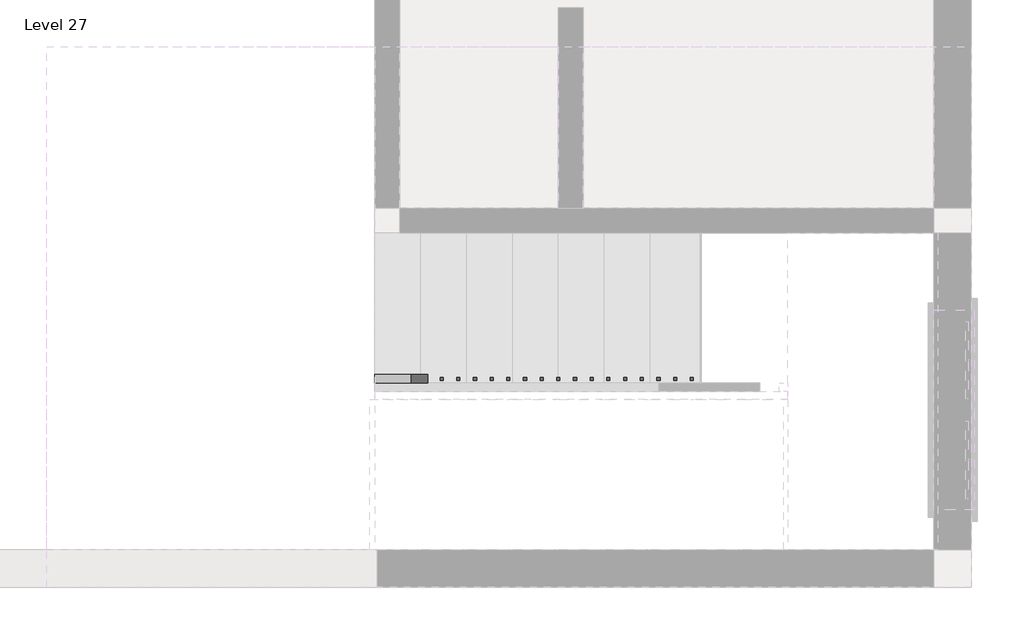
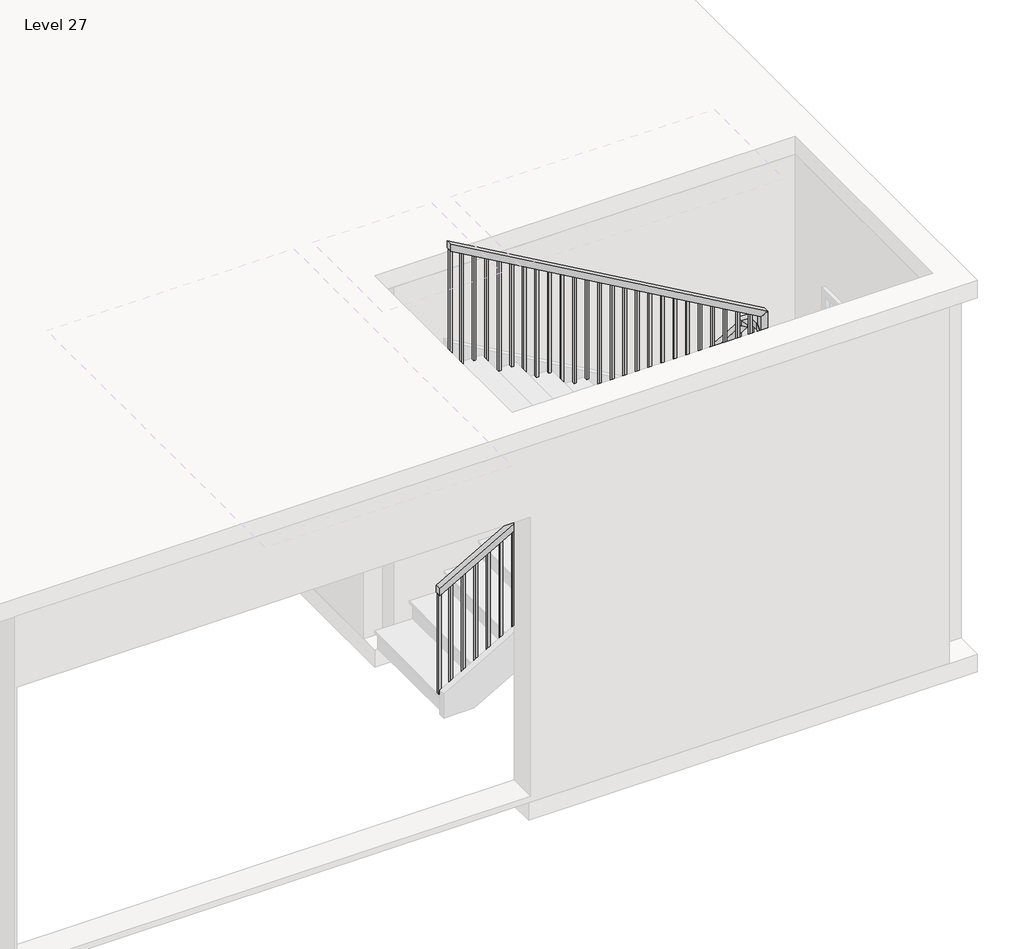
# One storey, part 2 of 3: 2 railings.
"""IFC4 building model written with IfcOpenShell, lengths in millimetres."""

from ifc_helpers import new_model, si_unit, frame, origin, place, context, project, spatial, polyline, outline, extrude, faceted_brep, element, save

model = new_model("IFC4")

# Units and contexts
model_context = context("Model", 3, world=origin())
ifc_project = project(units=[si_unit("LENGTHUNIT", "METRE", prefix="MILLI")], contexts=[model_context])

# Site, building, storey
site = spatial("IfcSite", under=ifc_project)
building = spatial("IfcBuilding", under=site)
storey = spatial("IfcBuildingStorey", under=building, Name="Level 27", Elevation=22402.8)

# Railings
placement = place(None, origin())
element("IfcRailing", 1, ObjectType="Handrail - Rectangular", at=placement, inside=storey, context=model_context, shape_type="SolidModel", body=[
    faceted_brep([(-1591.1154463, -4686.5544725, 23477.22), (-1591.1154463, -4686.5544725, 23418.6782835), (-1591.1154463, -4737.3544725, 23418.6782835), (-1591.1154463, -4737.3544725, 23477.22), (847.2845537, -4686.5544725, 24873.7581818), (898.0845537, -4686.5544725, 24844.3110107), (898.0845537, -4737.3544725, 24844.3110107), (847.2845537, -4737.3544725, 24873.7581818), (847.2845537, -4686.5544725, 24917.4), (898.0845537, -4686.5544725, 24866.6), (898.0845537, -4737.3544725, 24866.6), (847.2845537, -4737.3544725, 24917.4), (974.2845537, -4686.5544725, 24917.4), (974.2845537, -4686.5544725, 24866.6), (923.4845537, -4737.3544725, 24866.6), (923.4845537, -4737.3544725, 24917.4), (974.2845537, -4813.5544725, 24917.4), (974.2845537, -4813.5544725, 24866.6), (923.4845537, -4813.5544725, 24866.6), (923.4845537, -4813.5544725, 24917.4), (974.2845537, -4838.9544725, 24917.4), (923.4845537, -4838.9544725, 24917.4), (923.4845537, -4889.7544725, 24866.6), (974.2845537, -4889.7544725, 24866.6)], [[[0, 1, 2, 3]], [[1, 0, 4, 5]], [[2, 1, 5, 6]], [[3, 2, 6, 7]], [[0, 3, 7, 4]], [[5, 4, 8, 9]], [[6, 5, 9, 10]], [[7, 6, 10, 11]], [[4, 7, 11, 8]], [[9, 8, 12, 13]], [[10, 9, 13, 14]], [[11, 10, 14, 15]], [[8, 11, 15, 12]], [[13, 12, 16, 17]], [[14, 13, 17, 18]], [[15, 14, 18, 19]], [[12, 15, 19, 16]], [[20, 21, 22, 23]], [[17, 16, 20, 23]], [[18, 17, 23, 22]], [[19, 18, 22, 21]], [[16, 19, 21, 20]]]),
    faceted_brep([(974.2845537, -4838.9544725, 24917.4), (974.2845537, -4889.7544725, 24866.6), (923.4845537, -4889.7544725, 24866.6), (923.4845537, -4838.9544725, 24917.4), (974.2845537, -4838.9544725, 25048.3254545), (923.4845537, -4838.9544725, 25018.8782835), (923.4845537, -4889.7544725, 25018.8782835), (974.2845537, -4889.7544725, 25048.3254545)], [[[0, 1, 2, 3]], [[4, 5, 6, 7]], [[1, 0, 4, 7]], [[2, 1, 7, 6]], [[3, 2, 6, 5]], [[0, 3, 5, 4]]]),
    faceted_brep([(974.2845537, -4889.7544725, 25048.3254545), (923.4845537, -4889.7544725, 25018.8782835), (923.4845537, -4838.9544725, 25018.8782835), (974.2845537, -4838.9544725, 25048.3254545), (-1591.1154463, -4889.7544725, 26517.6), (-1591.1154463, -4838.9544725, 26517.6), (-1591.1154463, -4838.9544725, 26459.0582835), (-1591.1154463, -4889.7544725, 26459.0582835)], [[[0, 1, 2, 3]], [[4, 5, 6, 7]], [[1, 0, 4, 7]], [[2, 1, 7, 6]], [[3, 2, 6, 5]], [[0, 3, 5, 4]]]),
    extrude(outline(polyline([(26395.4139653, -1479.9904463), (26406.3244198, -1499.0404463), (25443.18, -1499.0404463), (25443.18, -1479.9904463), (26395.4139653, -1479.9904463)])), frame((0.0, -4873.8794725, 0.0), z_axis=(0.0, 1.0, 0.0), x_axis=(0.0, 0.0, 1.0)), (0.0, 0.0, 1.0), 19.05),
    extrude(outline(polyline([(26337.2248744, -1378.3904463), (26348.1353289, -1397.4404463), (25443.18, -1397.4404463), (25443.18, -1378.3904463), (26337.2248744, -1378.3904463)])), frame((0.0, -4873.8794725, 0.0), z_axis=(0.0, 1.0, 0.0), x_axis=(0.0, 0.0, 1.0)), (0.0, 0.0, 1.0), 19.05),
    extrude(outline(polyline([(26279.0357835, -1276.7904463), (26289.946238, -1295.8404463), (25283.16, -1295.8404463), (25283.16, -1276.7904463), (26279.0357835, -1276.7904463)])), frame((0.0, -4873.8794725, 0.0), z_axis=(0.0, 1.0, 0.0), x_axis=(0.0, 0.0, 1.0)), (0.0, 0.0, 1.0), 19.05),
    extrude(outline(polyline([(26220.8466926, -1175.1904463), (26231.7571471, -1194.2404463), (25283.16, -1194.2404463), (25283.16, -1175.1904463), (26220.8466926, -1175.1904463)])), frame((0.0, -4873.8794725, 0.0), z_axis=(0.0, 1.0, 0.0), x_axis=(0.0, 0.0, 1.0)), (0.0, 0.0, 1.0), 19.05),
    extrude(outline(polyline([(26162.6576016, -1073.5904463), (26173.5680562, -1092.6404463), (25283.16, -1092.6404463), (25283.16, -1073.5904463), (26162.6576016, -1073.5904463)])), frame((0.0, -4873.8794725, 0.0), z_axis=(0.0, 1.0, 0.0), x_axis=(0.0, 0.0, 1.0)), (0.0, 0.0, 1.0), 19.05),
    extrude(outline(polyline([(26104.4685107, -971.9904463), (26115.3789653, -991.0404463), (25123.14, -991.0404463), (25123.14, -971.9904463), (26104.4685107, -971.9904463)])), frame((0.0, -4873.8794725, 0.0), z_axis=(0.0, 1.0, 0.0), x_axis=(0.0, 0.0, 1.0)), (0.0, 0.0, 1.0), 19.05),
    extrude(outline(polyline([(26046.2794198, -870.3904463), (26057.1898744, -889.4404463), (25123.14, -889.4404463), (25123.14, -870.3904463), (26046.2794198, -870.3904463)])), frame((0.0, -4873.8794725, 0.0), z_axis=(0.0, 1.0, 0.0), x_axis=(0.0, 0.0, 1.0)), (0.0, 0.0, 1.0), 19.05),
    extrude(outline(polyline([(25988.0903289, -768.7904463), (25999.0007835, -787.8404463), (25123.14, -787.8404463), (25123.14, -768.7904463), (25988.0903289, -768.7904463)])), frame((0.0, -4873.8794725, 0.0), z_axis=(0.0, 1.0, 0.0), x_axis=(0.0, 0.0, 1.0)), (0.0, 0.0, 1.0), 19.05),
    extrude(outline(polyline([(25929.901238, -667.1904463), (25940.8116926, -686.2404463), (24963.12, -686.2404463), (24963.12, -667.1904463), (25929.901238, -667.1904463)])), frame((0.0, -4873.8794725, 0.0), z_axis=(0.0, 1.0, 0.0), x_axis=(0.0, 0.0, 1.0)), (0.0, 0.0, 1.0), 19.05),
    extrude(outline(polyline([(25871.7121471, -565.5904463), (25882.6226016, -584.6404463), (24963.12, -584.6404463), (24963.12, -565.5904463), (25871.7121471, -565.5904463)])), frame((0.0, -4873.8794725, 0.0), z_axis=(0.0, 1.0, 0.0), x_axis=(0.0, 0.0, 1.0)), (0.0, 0.0, 1.0), 19.05),
    extrude(outline(polyline([(25813.5230562, -463.9904463), (25824.4335107, -483.0404463), (24963.12, -483.0404463), (24963.12, -463.9904463), (25813.5230562, -463.9904463)])), frame((0.0, -4873.8794725, 0.0), z_axis=(0.0, 1.0, 0.0), x_axis=(0.0, 0.0, 1.0)), (0.0, 0.0, 1.0), 19.05),
    extrude(outline(polyline([(25755.3339653, -362.3904463), (25766.2444198, -381.4404463), (24803.1, -381.4404463), (24803.1, -362.3904463), (25755.3339653, -362.3904463)])), frame((0.0, -4873.8794725, 0.0), z_axis=(0.0, 1.0, 0.0), x_axis=(0.0, 0.0, 1.0)), (0.0, 0.0, 1.0), 19.05),
    extrude(outline(polyline([(25697.1448744, -260.7904463), (25708.0553289, -279.8404463), (24803.1, -279.8404463), (24803.1, -260.7904463), (25697.1448744, -260.7904463)])), frame((0.0, -4873.8794725, 0.0), z_axis=(0.0, 1.0, 0.0), x_axis=(0.0, 0.0, 1.0)), (0.0, 0.0, 1.0), 19.05),
    extrude(outline(polyline([(25638.9557835, -159.1904463), (25649.866238, -178.2404463), (24643.08, -178.2404463), (24643.08, -159.1904463), (25638.9557835, -159.1904463)])), frame((0.0, -4873.8794725, 0.0), z_axis=(0.0, 1.0, 0.0), x_axis=(0.0, 0.0, 1.0)), (0.0, 0.0, 1.0), 19.05),
    extrude(outline(polyline([(25580.7666926, -57.5904463), (25591.6771471, -76.6404463), (24643.08, -76.6404463), (24643.08, -57.5904463), (25580.7666926, -57.5904463)])), frame((0.0, -4873.8794725, 0.0), z_axis=(0.0, 1.0, 0.0), x_axis=(0.0, 0.0, 1.0)), (0.0, 0.0, 1.0), 19.05),
    extrude(outline(polyline([(25522.5776016, 44.0095537), (25533.4880562, 24.9595537), (24643.08, 24.9595537), (24643.08, 44.0095537), (25522.5776016, 44.0095537)])), frame((0.0, -4873.8794725, 0.0), z_axis=(0.0, 1.0, 0.0), x_axis=(0.0, 0.0, 1.0)), (0.0, 0.0, 1.0), 19.05),
    extrude(outline(polyline([(25464.3885107, 145.6095537), (25475.2989653, 126.5595537), (24483.06, 126.5595537), (24483.06, 145.6095537), (25464.3885107, 145.6095537)])), frame((0.0, -4873.8794725, 0.0), z_axis=(0.0, 1.0, 0.0), x_axis=(0.0, 0.0, 1.0)), (0.0, 0.0, 1.0), 19.05),
    extrude(outline(polyline([(25406.1994198, 247.2095537), (25417.1098744, 228.1595537), (24483.06, 228.1595537), (24483.06, 247.2095537), (25406.1994198, 247.2095537)])), frame((0.0, -4873.8794725, 0.0), z_axis=(0.0, 1.0, 0.0), x_axis=(0.0, 0.0, 1.0)), (0.0, 0.0, 1.0), 19.05),
    extrude(outline(polyline([(25348.0103289, 348.8095537), (25358.9207835, 329.7595537), (24483.06, 329.7595537), (24483.06, 348.8095537), (25348.0103289, 348.8095537)])), frame((0.0, -4873.8794725, 0.0), z_axis=(0.0, 1.0, 0.0), x_axis=(0.0, 0.0, 1.0)), (0.0, 0.0, 1.0), 19.05),
    extrude(outline(polyline([(25289.821238, 450.4095537), (25300.7316926, 431.3595537), (24323.04, 431.3595537), (24323.04, 450.4095537), (25289.821238, 450.4095537)])), frame((0.0, -4873.8794725, 0.0), z_axis=(0.0, 1.0, 0.0), x_axis=(0.0, 0.0, 1.0)), (0.0, 0.0, 1.0), 19.05),
    extrude(outline(polyline([(25231.6321471, 552.0095537), (25242.5426016, 532.9595537), (24323.04, 532.9595537), (24323.04, 552.0095537), (25231.6321471, 552.0095537)])), frame((0.0, -4873.8794725, 0.0), z_axis=(0.0, 1.0, 0.0), x_axis=(0.0, 0.0, 1.0)), (0.0, 0.0, 1.0), 19.05),
    extrude(outline(polyline([(25173.4430562, 653.6095537), (25184.3535107, 634.5595537), (24323.04, 634.5595537), (24323.04, 653.6095537), (25173.4430562, 653.6095537)])), frame((0.0, -4873.8794725, 0.0), z_axis=(0.0, 1.0, 0.0), x_axis=(0.0, 0.0, 1.0)), (0.0, 0.0, 1.0), 19.05),
    extrude(outline(polyline([(25115.2539653, 755.2095537), (25126.1644198, 736.1595537), (24163.02, 736.1595537), (24163.02, 755.2095537), (25115.2539653, 755.2095537)])), frame((0.0, -4873.8794725, 0.0), z_axis=(0.0, 1.0, 0.0), x_axis=(0.0, 0.0, 1.0)), (0.0, 0.0, 1.0), 19.05),
    extrude(outline(polyline([(25057.0648744, 856.8095537), (25067.9753289, 837.7595537), (24163.02, 837.7595537), (24163.02, 856.8095537), (25057.0648744, 856.8095537)])), frame((0.0, -4873.8794725, 0.0), z_axis=(0.0, 1.0, 0.0), x_axis=(0.0, 0.0, 1.0)), (0.0, 0.0, 1.0), 19.05),
    extrude(outline(polyline([(939.3595537, -4804.0294725), (958.4095537, -4804.0294725), (958.4095537, -4823.0794725), (939.3595537, -4823.0794725), (939.3595537, -4804.0294725)])), frame((0.0, 0.0, 24003.0), z_axis=(0.0, 0.0, 1.0), x_axis=(1.0, 0.0, 0.0)), (0.0, 0.0, 1.0), 863.6),
    extrude(outline(polyline([(24820.6716926, 856.8095537), (24809.761238, 837.7595537), (23842.98, 837.7595537), (23842.98, 856.8095537), (24820.6716926, 856.8095537)])), frame((0.0, -4721.4794725, 0.0), z_axis=(0.0, 1.0, 0.0), x_axis=(0.0, 0.0, 1.0)), (0.0, 0.0, 1.0), 19.05),
    extrude(outline(polyline([(24762.4826016, 755.2095537), (24751.5721471, 736.1595537), (23842.98, 736.1595537), (23842.98, 755.2095537), (24762.4826016, 755.2095537)])), frame((0.0, -4721.4794725, 0.0), z_axis=(0.0, 1.0, 0.0), x_axis=(0.0, 0.0, 1.0)), (0.0, 0.0, 1.0), 19.05),
    extrude(outline(polyline([(24704.2935107, 653.6095537), (24693.3830562, 634.5595537), (23842.98, 634.5595537), (23842.98, 653.6095537), (24704.2935107, 653.6095537)])), frame((0.0, -4721.4794725, 0.0), z_axis=(0.0, 1.0, 0.0), x_axis=(0.0, 0.0, 1.0)), (0.0, 0.0, 1.0), 19.05),
    extrude(outline(polyline([(24646.1044198, 552.0095537), (24635.1939653, 532.9595537), (23682.96, 532.9595537), (23682.96, 552.0095537), (24646.1044198, 552.0095537)])), frame((0.0, -4721.4794725, 0.0), z_axis=(0.0, 1.0, 0.0), x_axis=(0.0, 0.0, 1.0)), (0.0, 0.0, 1.0), 19.05),
    extrude(outline(polyline([(24587.9153289, 450.4095537), (24577.0048744, 431.3595537), (23682.96, 431.3595537), (23682.96, 450.4095537), (24587.9153289, 450.4095537)])), frame((0.0, -4721.4794725, 0.0), z_axis=(0.0, 1.0, 0.0), x_axis=(0.0, 0.0, 1.0)), (0.0, 0.0, 1.0), 19.05),
    extrude(outline(polyline([(24529.726238, 348.8095537), (24518.8157835, 329.7595537), (23522.94, 329.7595537), (23522.94, 348.8095537), (24529.726238, 348.8095537)])), frame((0.0, -4721.4794725, 0.0), z_axis=(0.0, 1.0, 0.0), x_axis=(0.0, 0.0, 1.0)), (0.0, 0.0, 1.0), 19.05),
    extrude(outline(polyline([(24471.5371471, 247.2095537), (24460.6266926, 228.1595537), (23522.94, 228.1595537), (23522.94, 247.2095537), (24471.5371471, 247.2095537)])), frame((0.0, -4721.4794725, 0.0), z_axis=(0.0, 1.0, 0.0), x_axis=(0.0, 0.0, 1.0)), (0.0, 0.0, 1.0), 19.05),
    extrude(outline(polyline([(24413.3480562, 145.6095537), (24402.4376016, 126.5595537), (23522.94, 126.5595537), (23522.94, 145.6095537), (24413.3480562, 145.6095537)])), frame((0.0, -4721.4794725, 0.0), z_axis=(0.0, 1.0, 0.0), x_axis=(0.0, 0.0, 1.0)), (0.0, 0.0, 1.0), 19.05),
    extrude(outline(polyline([(24355.1589653, 44.0095537), (24344.2485107, 24.9595537), (23362.92, 24.9595537), (23362.92, 44.0095537), (24355.1589653, 44.0095537)])), frame((0.0, -4721.4794725, 0.0), z_axis=(0.0, 1.0, 0.0), x_axis=(0.0, 0.0, 1.0)), (0.0, 0.0, 1.0), 19.05),
    extrude(outline(polyline([(24296.9698744, -57.5904463), (24286.0594198, -76.6404463), (23362.92, -76.6404463), (23362.92, -57.5904463), (24296.9698744, -57.5904463)])), frame((0.0, -4721.4794725, 0.0), z_axis=(0.0, 1.0, 0.0), x_axis=(0.0, 0.0, 1.0)), (0.0, 0.0, 1.0), 19.05),
    extrude(outline(polyline([(24238.7807835, -159.1904463), (24227.8703289, -178.2404463), (23362.92, -178.2404463), (23362.92, -159.1904463), (24238.7807835, -159.1904463)])), frame((0.0, -4721.4794725, 0.0), z_axis=(0.0, 1.0, 0.0), x_axis=(0.0, 0.0, 1.0)), (0.0, 0.0, 1.0), 19.05),
    extrude(outline(polyline([(24180.5916926, -260.7904463), (24169.681238, -279.8404463), (23202.9, -279.8404463), (23202.9, -260.7904463), (24180.5916926, -260.7904463)])), frame((0.0, -4721.4794725, 0.0), z_axis=(0.0, 1.0, 0.0), x_axis=(0.0, 0.0, 1.0)), (0.0, 0.0, 1.0), 19.05),
    extrude(outline(polyline([(24122.4026016, -362.3904463), (24111.4921471, -381.4404463), (23202.9, -381.4404463), (23202.9, -362.3904463), (24122.4026016, -362.3904463)])), frame((0.0, -4721.4794725, 0.0), z_axis=(0.0, 1.0, 0.0), x_axis=(0.0, 0.0, 1.0)), (0.0, 0.0, 1.0), 19.05),
    extrude(outline(polyline([(24064.2135107, -463.9904463), (24053.3030562, -483.0404463), (23202.9, -483.0404463), (23202.9, -463.9904463), (24064.2135107, -463.9904463)])), frame((0.0, -4721.4794725, 0.0), z_axis=(0.0, 1.0, 0.0), x_axis=(0.0, 0.0, 1.0)), (0.0, 0.0, 1.0), 19.05),
    extrude(outline(polyline([(24006.0244198, -565.5904463), (23995.1139653, -584.6404463), (23042.88, -584.6404463), (23042.88, -565.5904463), (24006.0244198, -565.5904463)])), frame((0.0, -4721.4794725, 0.0), z_axis=(0.0, 1.0, 0.0), x_axis=(0.0, 0.0, 1.0)), (0.0, 0.0, 1.0), 19.05),
    extrude(outline(polyline([(23947.8353289, -667.1904463), (23936.9248744, -686.2404463), (23042.88, -686.2404463), (23042.88, -667.1904463), (23947.8353289, -667.1904463)])), frame((0.0, -4721.4794725, 0.0), z_axis=(0.0, 1.0, 0.0), x_axis=(0.0, 0.0, 1.0)), (0.0, 0.0, 1.0), 19.05),
    extrude(outline(polyline([(23889.646238, -768.7904463), (23878.7357835, -787.8404463), (22882.86, -787.8404463), (22882.86, -768.7904463), (23889.646238, -768.7904463)])), frame((0.0, -4721.4794725, 0.0), z_axis=(0.0, 1.0, 0.0), x_axis=(0.0, 0.0, 1.0)), (0.0, 0.0, 1.0), 19.05),
    extrude(outline(polyline([(23831.4571471, -870.3904463), (23820.5466926, -889.4404463), (22882.86, -889.4404463), (22882.86, -870.3904463), (23831.4571471, -870.3904463)])), frame((0.0, -4721.4794725, 0.0), z_axis=(0.0, 1.0, 0.0), x_axis=(0.0, 0.0, 1.0)), (0.0, 0.0, 1.0), 19.05),
    extrude(outline(polyline([(23773.2680562, -971.9904463), (23762.3576016, -991.0404463), (22882.86, -991.0404463), (22882.86, -971.9904463), (23773.2680562, -971.9904463)])), frame((0.0, -4721.4794725, 0.0), z_axis=(0.0, 1.0, 0.0), x_axis=(0.0, 0.0, 1.0)), (0.0, 0.0, 1.0), 19.05),
    extrude(outline(polyline([(23715.0789653, -1073.5904463), (23704.1685107, -1092.6404463), (22722.84, -1092.6404463), (22722.84, -1073.5904463), (23715.0789653, -1073.5904463)])), frame((0.0, -4721.4794725, 0.0), z_axis=(0.0, 1.0, 0.0), x_axis=(0.0, 0.0, 1.0)), (0.0, 0.0, 1.0), 19.05),
    extrude(outline(polyline([(23656.8898744, -1175.1904463), (23645.9794198, -1194.2404463), (22722.84, -1194.2404463), (22722.84, -1175.1904463), (23656.8898744, -1175.1904463)])), frame((0.0, -4721.4794725, 0.0), z_axis=(0.0, 1.0, 0.0), x_axis=(0.0, 0.0, 1.0)), (0.0, 0.0, 1.0), 19.05),
    extrude(outline(polyline([(23598.7007835, -1276.7904463), (23587.7903289, -1295.8404463), (22722.84, -1295.8404463), (22722.84, -1276.7904463), (23598.7007835, -1276.7904463)])), frame((0.0, -4721.4794725, 0.0), z_axis=(0.0, 1.0, 0.0), x_axis=(0.0, 0.0, 1.0)), (0.0, 0.0, 1.0), 19.05),
    extrude(outline(polyline([(23540.5116926, -1378.3904463), (23529.601238, -1397.4404463), (22562.82, -1397.4404463), (22562.82, -1378.3904463), (23540.5116926, -1378.3904463)])), frame((0.0, -4721.4794725, 0.0), z_axis=(0.0, 1.0, 0.0), x_axis=(0.0, 0.0, 1.0)), (0.0, 0.0, 1.0), 19.05),
    extrude(outline(polyline([(23482.3226016, -1479.9904463), (23471.4121471, -1499.0404463), (22562.82, -1499.0404463), (22562.82, -1479.9904463), (23482.3226016, -1479.9904463)])), frame((0.0, -4721.4794725, 0.0), z_axis=(0.0, 1.0, 0.0), x_axis=(0.0, 0.0, 1.0)), (0.0, 0.0, 1.0), 19.05),
    extrude(outline(polyline([(939.3595537, -4854.8294725), (958.4095537, -4854.8294725), (958.4095537, -4873.8794725), (939.3595537, -4873.8794725), (939.3595537, -4854.8294725)])), frame((0.0, 0.0, 24003.0), z_axis=(0.0, 0.0, 1.0), x_axis=(1.0, 0.0, 0.0)), (0.0, 0.0, 1.0), 863.6),
    extrude(outline(polyline([(939.3595537, -4721.4794725), (939.3595537, -4702.4294725), (958.4095537, -4702.4294725), (958.4095537, -4721.4794725), (939.3595537, -4721.4794725)])), frame((0.0, 0.0, 24003.0), z_axis=(0.0, 0.0, 1.0), x_axis=(1.0, 0.0, 0.0)), (0.0, 0.0, 1.0), 863.6),
    extrude(outline(polyline([(26448.1478289, -1572.0654463), (26459.0582835, -1591.1154463), (25443.18, -1591.1154463), (25443.18, -1572.0654463), (26448.1478289, -1572.0654463)])), frame((0.0, -4873.8794725, 0.0), z_axis=(0.0, 1.0, 0.0), x_axis=(0.0, 0.0, 1.0)), (0.0, 0.0, 1.0), 19.05),
    extrude(outline(polyline([(23429.588738, -1572.0654463), (23418.6782835, -1591.1154463), (22562.82, -1591.1154463), (22562.82, -1572.0654463), (23429.588738, -1572.0654463)])), frame((0.0, -4721.4794725, 0.0), z_axis=(0.0, 1.0, 0.0), x_axis=(0.0, 0.0, 1.0)), (0.0, 0.0, 1.0), 19.05),
])
element("IfcRailing", 2, ObjectType="Handrail - Rectangular", at=placement, inside=storey, context=model_context, shape_type="SolidModel", body=[
    faceted_brep([(-1591.1154463, -4686.5544725, 23477.22), (-1591.1154463, -4686.5544725, 23418.6782835), (-1591.1154463, -4737.3544725, 23418.6782835), (-1591.1154463, -4737.3544725, 23477.22), (847.2845537, -4686.5544725, 24873.7581818), (898.0845537, -4686.5544725, 24844.3110107), (898.0845537, -4737.3544725, 24844.3110107), (847.2845537, -4737.3544725, 24873.7581818), (847.2845537, -4686.5544725, 24917.4), (898.0845537, -4686.5544725, 24866.6), (898.0845537, -4737.3544725, 24866.6), (847.2845537, -4737.3544725, 24917.4), (974.2845537, -4686.5544725, 24917.4), (974.2845537, -4686.5544725, 24866.6), (923.4845537, -4737.3544725, 24866.6), (923.4845537, -4737.3544725, 24917.4), (974.2845537, -4813.5544725, 24917.4), (974.2845537, -4813.5544725, 24866.6), (923.4845537, -4813.5544725, 24866.6), (923.4845537, -4813.5544725, 24917.4), (974.2845537, -4838.9544725, 24917.4), (923.4845537, -4838.9544725, 24917.4), (923.4845537, -4889.7544725, 24866.6), (974.2845537, -4889.7544725, 24866.6)], [[[0, 1, 2, 3]], [[1, 0, 4, 5]], [[2, 1, 5, 6]], [[3, 2, 6, 7]], [[0, 3, 7, 4]], [[5, 4, 8, 9]], [[6, 5, 9, 10]], [[7, 6, 10, 11]], [[4, 7, 11, 8]], [[9, 8, 12, 13]], [[10, 9, 13, 14]], [[11, 10, 14, 15]], [[8, 11, 15, 12]], [[13, 12, 16, 17]], [[14, 13, 17, 18]], [[15, 14, 18, 19]], [[12, 15, 19, 16]], [[20, 21, 22, 23]], [[17, 16, 20, 23]], [[18, 17, 23, 22]], [[19, 18, 22, 21]], [[16, 19, 21, 20]]]),
    faceted_brep([(974.2845537, -4838.9544725, 24917.4), (974.2845537, -4889.7544725, 24866.6), (923.4845537, -4889.7544725, 24866.6), (923.4845537, -4838.9544725, 24917.4), (974.2845537, -4838.9544725, 25048.3254545), (923.4845537, -4838.9544725, 25018.8782835), (923.4845537, -4889.7544725, 25018.8782835), (974.2845537, -4889.7544725, 25048.3254545)], [[[0, 1, 2, 3]], [[4, 5, 6, 7]], [[1, 0, 4, 7]], [[2, 1, 7, 6]], [[3, 2, 6, 5]], [[0, 3, 5, 4]]]),
    faceted_brep([(974.2845537, -4889.7544725, 25048.3254545), (923.4845537, -4889.7544725, 25018.8782835), (923.4845537, -4838.9544725, 25018.8782835), (974.2845537, -4838.9544725, 25048.3254545), (-1591.1154463, -4889.7544725, 26517.6), (-1591.1154463, -4838.9544725, 26517.6), (-1591.1154463, -4838.9544725, 26459.0582835), (-1591.1154463, -4889.7544725, 26459.0582835)], [[[0, 1, 2, 3]], [[4, 5, 6, 7]], [[1, 0, 4, 7]], [[2, 1, 7, 6]], [[3, 2, 6, 5]], [[0, 3, 5, 4]]]),
    extrude(outline(polyline([(26395.4139653, -1479.9904463), (26406.3244198, -1499.0404463), (25443.18, -1499.0404463), (25443.18, -1479.9904463), (26395.4139653, -1479.9904463)])), frame((0.0, -4873.8794725, 0.0), z_axis=(0.0, 1.0, 0.0), x_axis=(0.0, 0.0, 1.0)), (0.0, 0.0, 1.0), 19.05),
    extrude(outline(polyline([(26337.2248744, -1378.3904463), (26348.1353289, -1397.4404463), (25443.18, -1397.4404463), (25443.18, -1378.3904463), (26337.2248744, -1378.3904463)])), frame((0.0, -4873.8794725, 0.0), z_axis=(0.0, 1.0, 0.0), x_axis=(0.0, 0.0, 1.0)), (0.0, 0.0, 1.0), 19.05),
    extrude(outline(polyline([(26279.0357835, -1276.7904463), (26289.946238, -1295.8404463), (25283.16, -1295.8404463), (25283.16, -1276.7904463), (26279.0357835, -1276.7904463)])), frame((0.0, -4873.8794725, 0.0), z_axis=(0.0, 1.0, 0.0), x_axis=(0.0, 0.0, 1.0)), (0.0, 0.0, 1.0), 19.05),
    extrude(outline(polyline([(26220.8466926, -1175.1904463), (26231.7571471, -1194.2404463), (25283.16, -1194.2404463), (25283.16, -1175.1904463), (26220.8466926, -1175.1904463)])), frame((0.0, -4873.8794725, 0.0), z_axis=(0.0, 1.0, 0.0), x_axis=(0.0, 0.0, 1.0)), (0.0, 0.0, 1.0), 19.05),
    extrude(outline(polyline([(26162.6576016, -1073.5904463), (26173.5680562, -1092.6404463), (25283.16, -1092.6404463), (25283.16, -1073.5904463), (26162.6576016, -1073.5904463)])), frame((0.0, -4873.8794725, 0.0), z_axis=(0.0, 1.0, 0.0), x_axis=(0.0, 0.0, 1.0)), (0.0, 0.0, 1.0), 19.05),
    extrude(outline(polyline([(26104.4685107, -971.9904463), (26115.3789653, -991.0404463), (25123.14, -991.0404463), (25123.14, -971.9904463), (26104.4685107, -971.9904463)])), frame((0.0, -4873.8794725, 0.0), z_axis=(0.0, 1.0, 0.0), x_axis=(0.0, 0.0, 1.0)), (0.0, 0.0, 1.0), 19.05),
    extrude(outline(polyline([(26046.2794198, -870.3904463), (26057.1898744, -889.4404463), (25123.14, -889.4404463), (25123.14, -870.3904463), (26046.2794198, -870.3904463)])), frame((0.0, -4873.8794725, 0.0), z_axis=(0.0, 1.0, 0.0), x_axis=(0.0, 0.0, 1.0)), (0.0, 0.0, 1.0), 19.05),
    extrude(outline(polyline([(25988.0903289, -768.7904463), (25999.0007835, -787.8404463), (25123.14, -787.8404463), (25123.14, -768.7904463), (25988.0903289, -768.7904463)])), frame((0.0, -4873.8794725, 0.0), z_axis=(0.0, 1.0, 0.0), x_axis=(0.0, 0.0, 1.0)), (0.0, 0.0, 1.0), 19.05),
    extrude(outline(polyline([(25929.901238, -667.1904463), (25940.8116926, -686.2404463), (24963.12, -686.2404463), (24963.12, -667.1904463), (25929.901238, -667.1904463)])), frame((0.0, -4873.8794725, 0.0), z_axis=(0.0, 1.0, 0.0), x_axis=(0.0, 0.0, 1.0)), (0.0, 0.0, 1.0), 19.05),
    extrude(outline(polyline([(25871.7121471, -565.5904463), (25882.6226016, -584.6404463), (24963.12, -584.6404463), (24963.12, -565.5904463), (25871.7121471, -565.5904463)])), frame((0.0, -4873.8794725, 0.0), z_axis=(0.0, 1.0, 0.0), x_axis=(0.0, 0.0, 1.0)), (0.0, 0.0, 1.0), 19.05),
    extrude(outline(polyline([(25813.5230562, -463.9904463), (25824.4335107, -483.0404463), (24963.12, -483.0404463), (24963.12, -463.9904463), (25813.5230562, -463.9904463)])), frame((0.0, -4873.8794725, 0.0), z_axis=(0.0, 1.0, 0.0), x_axis=(0.0, 0.0, 1.0)), (0.0, 0.0, 1.0), 19.05),
    extrude(outline(polyline([(25755.3339653, -362.3904463), (25766.2444198, -381.4404463), (24803.1, -381.4404463), (24803.1, -362.3904463), (25755.3339653, -362.3904463)])), frame((0.0, -4873.8794725, 0.0), z_axis=(0.0, 1.0, 0.0), x_axis=(0.0, 0.0, 1.0)), (0.0, 0.0, 1.0), 19.05),
    extrude(outline(polyline([(25697.1448744, -260.7904463), (25708.0553289, -279.8404463), (24803.1, -279.8404463), (24803.1, -260.7904463), (25697.1448744, -260.7904463)])), frame((0.0, -4873.8794725, 0.0), z_axis=(0.0, 1.0, 0.0), x_axis=(0.0, 0.0, 1.0)), (0.0, 0.0, 1.0), 19.05),
    extrude(outline(polyline([(25638.9557835, -159.1904463), (25649.866238, -178.2404463), (24643.08, -178.2404463), (24643.08, -159.1904463), (25638.9557835, -159.1904463)])), frame((0.0, -4873.8794725, 0.0), z_axis=(0.0, 1.0, 0.0), x_axis=(0.0, 0.0, 1.0)), (0.0, 0.0, 1.0), 19.05),
    extrude(outline(polyline([(25580.7666926, -57.5904463), (25591.6771471, -76.6404463), (24643.08, -76.6404463), (24643.08, -57.5904463), (25580.7666926, -57.5904463)])), frame((0.0, -4873.8794725, 0.0), z_axis=(0.0, 1.0, 0.0), x_axis=(0.0, 0.0, 1.0)), (0.0, 0.0, 1.0), 19.05),
    extrude(outline(polyline([(25522.5776016, 44.0095537), (25533.4880562, 24.9595537), (24643.08, 24.9595537), (24643.08, 44.0095537), (25522.5776016, 44.0095537)])), frame((0.0, -4873.8794725, 0.0), z_axis=(0.0, 1.0, 0.0), x_axis=(0.0, 0.0, 1.0)), (0.0, 0.0, 1.0), 19.05),
    extrude(outline(polyline([(25464.3885107, 145.6095537), (25475.2989653, 126.5595537), (24483.06, 126.5595537), (24483.06, 145.6095537), (25464.3885107, 145.6095537)])), frame((0.0, -4873.8794725, 0.0), z_axis=(0.0, 1.0, 0.0), x_axis=(0.0, 0.0, 1.0)), (0.0, 0.0, 1.0), 19.05),
    extrude(outline(polyline([(25406.1994198, 247.2095537), (25417.1098744, 228.1595537), (24483.06, 228.1595537), (24483.06, 247.2095537), (25406.1994198, 247.2095537)])), frame((0.0, -4873.8794725, 0.0), z_axis=(0.0, 1.0, 0.0), x_axis=(0.0, 0.0, 1.0)), (0.0, 0.0, 1.0), 19.05),
    extrude(outline(polyline([(25348.0103289, 348.8095537), (25358.9207835, 329.7595537), (24483.06, 329.7595537), (24483.06, 348.8095537), (25348.0103289, 348.8095537)])), frame((0.0, -4873.8794725, 0.0), z_axis=(0.0, 1.0, 0.0), x_axis=(0.0, 0.0, 1.0)), (0.0, 0.0, 1.0), 19.05),
    extrude(outline(polyline([(25289.821238, 450.4095537), (25300.7316926, 431.3595537), (24323.04, 431.3595537), (24323.04, 450.4095537), (25289.821238, 450.4095537)])), frame((0.0, -4873.8794725, 0.0), z_axis=(0.0, 1.0, 0.0), x_axis=(0.0, 0.0, 1.0)), (0.0, 0.0, 1.0), 19.05),
    extrude(outline(polyline([(25231.6321471, 552.0095537), (25242.5426016, 532.9595537), (24323.04, 532.9595537), (24323.04, 552.0095537), (25231.6321471, 552.0095537)])), frame((0.0, -4873.8794725, 0.0), z_axis=(0.0, 1.0, 0.0), x_axis=(0.0, 0.0, 1.0)), (0.0, 0.0, 1.0), 19.05),
    extrude(outline(polyline([(25173.4430562, 653.6095537), (25184.3535107, 634.5595537), (24323.04, 634.5595537), (24323.04, 653.6095537), (25173.4430562, 653.6095537)])), frame((0.0, -4873.8794725, 0.0), z_axis=(0.0, 1.0, 0.0), x_axis=(0.0, 0.0, 1.0)), (0.0, 0.0, 1.0), 19.05),
    extrude(outline(polyline([(25115.2539653, 755.2095537), (25126.1644198, 736.1595537), (24163.02, 736.1595537), (24163.02, 755.2095537), (25115.2539653, 755.2095537)])), frame((0.0, -4873.8794725, 0.0), z_axis=(0.0, 1.0, 0.0), x_axis=(0.0, 0.0, 1.0)), (0.0, 0.0, 1.0), 19.05),
    extrude(outline(polyline([(25057.0648744, 856.8095537), (25067.9753289, 837.7595537), (24163.02, 837.7595537), (24163.02, 856.8095537), (25057.0648744, 856.8095537)])), frame((0.0, -4873.8794725, 0.0), z_axis=(0.0, 1.0, 0.0), x_axis=(0.0, 0.0, 1.0)), (0.0, 0.0, 1.0), 19.05),
    extrude(outline(polyline([(939.3595537, -4804.0294725), (958.4095537, -4804.0294725), (958.4095537, -4823.0794725), (939.3595537, -4823.0794725), (939.3595537, -4804.0294725)])), frame((0.0, 0.0, 24003.0), z_axis=(0.0, 0.0, 1.0), x_axis=(1.0, 0.0, 0.0)), (0.0, 0.0, 1.0), 863.6),
    extrude(outline(polyline([(24820.6716926, 856.8095537), (24809.761238, 837.7595537), (23842.98, 837.7595537), (23842.98, 856.8095537), (24820.6716926, 856.8095537)])), frame((0.0, -4721.4794725, 0.0), z_axis=(0.0, 1.0, 0.0), x_axis=(0.0, 0.0, 1.0)), (0.0, 0.0, 1.0), 19.05),
    extrude(outline(polyline([(24762.4826016, 755.2095537), (24751.5721471, 736.1595537), (23842.98, 736.1595537), (23842.98, 755.2095537), (24762.4826016, 755.2095537)])), frame((0.0, -4721.4794725, 0.0), z_axis=(0.0, 1.0, 0.0), x_axis=(0.0, 0.0, 1.0)), (0.0, 0.0, 1.0), 19.05),
    extrude(outline(polyline([(24704.2935107, 653.6095537), (24693.3830562, 634.5595537), (23842.98, 634.5595537), (23842.98, 653.6095537), (24704.2935107, 653.6095537)])), frame((0.0, -4721.4794725, 0.0), z_axis=(0.0, 1.0, 0.0), x_axis=(0.0, 0.0, 1.0)), (0.0, 0.0, 1.0), 19.05),
    extrude(outline(polyline([(24646.1044198, 552.0095537), (24635.1939653, 532.9595537), (23682.96, 532.9595537), (23682.96, 552.0095537), (24646.1044198, 552.0095537)])), frame((0.0, -4721.4794725, 0.0), z_axis=(0.0, 1.0, 0.0), x_axis=(0.0, 0.0, 1.0)), (0.0, 0.0, 1.0), 19.05),
    extrude(outline(polyline([(24587.9153289, 450.4095537), (24577.0048744, 431.3595537), (23682.96, 431.3595537), (23682.96, 450.4095537), (24587.9153289, 450.4095537)])), frame((0.0, -4721.4794725, 0.0), z_axis=(0.0, 1.0, 0.0), x_axis=(0.0, 0.0, 1.0)), (0.0, 0.0, 1.0), 19.05),
    extrude(outline(polyline([(24529.726238, 348.8095537), (24518.8157835, 329.7595537), (23522.94, 329.7595537), (23522.94, 348.8095537), (24529.726238, 348.8095537)])), frame((0.0, -4721.4794725, 0.0), z_axis=(0.0, 1.0, 0.0), x_axis=(0.0, 0.0, 1.0)), (0.0, 0.0, 1.0), 19.05),
    extrude(outline(polyline([(24471.5371471, 247.2095537), (24460.6266926, 228.1595537), (23522.94, 228.1595537), (23522.94, 247.2095537), (24471.5371471, 247.2095537)])), frame((0.0, -4721.4794725, 0.0), z_axis=(0.0, 1.0, 0.0), x_axis=(0.0, 0.0, 1.0)), (0.0, 0.0, 1.0), 19.05),
    extrude(outline(polyline([(24413.3480562, 145.6095537), (24402.4376016, 126.5595537), (23522.94, 126.5595537), (23522.94, 145.6095537), (24413.3480562, 145.6095537)])), frame((0.0, -4721.4794725, 0.0), z_axis=(0.0, 1.0, 0.0), x_axis=(0.0, 0.0, 1.0)), (0.0, 0.0, 1.0), 19.05),
    extrude(outline(polyline([(24355.1589653, 44.0095537), (24344.2485107, 24.9595537), (23362.92, 24.9595537), (23362.92, 44.0095537), (24355.1589653, 44.0095537)])), frame((0.0, -4721.4794725, 0.0), z_axis=(0.0, 1.0, 0.0), x_axis=(0.0, 0.0, 1.0)), (0.0, 0.0, 1.0), 19.05),
    extrude(outline(polyline([(24296.9698744, -57.5904463), (24286.0594198, -76.6404463), (23362.92, -76.6404463), (23362.92, -57.5904463), (24296.9698744, -57.5904463)])), frame((0.0, -4721.4794725, 0.0), z_axis=(0.0, 1.0, 0.0), x_axis=(0.0, 0.0, 1.0)), (0.0, 0.0, 1.0), 19.05),
    extrude(outline(polyline([(24238.7807835, -159.1904463), (24227.8703289, -178.2404463), (23362.92, -178.2404463), (23362.92, -159.1904463), (24238.7807835, -159.1904463)])), frame((0.0, -4721.4794725, 0.0), z_axis=(0.0, 1.0, 0.0), x_axis=(0.0, 0.0, 1.0)), (0.0, 0.0, 1.0), 19.05),
    extrude(outline(polyline([(24180.5916926, -260.7904463), (24169.681238, -279.8404463), (23202.9, -279.8404463), (23202.9, -260.7904463), (24180.5916926, -260.7904463)])), frame((0.0, -4721.4794725, 0.0), z_axis=(0.0, 1.0, 0.0), x_axis=(0.0, 0.0, 1.0)), (0.0, 0.0, 1.0), 19.05),
    extrude(outline(polyline([(24122.4026016, -362.3904463), (24111.4921471, -381.4404463), (23202.9, -381.4404463), (23202.9, -362.3904463), (24122.4026016, -362.3904463)])), frame((0.0, -4721.4794725, 0.0), z_axis=(0.0, 1.0, 0.0), x_axis=(0.0, 0.0, 1.0)), (0.0, 0.0, 1.0), 19.05),
    extrude(outline(polyline([(24064.2135107, -463.9904463), (24053.3030562, -483.0404463), (23202.9, -483.0404463), (23202.9, -463.9904463), (24064.2135107, -463.9904463)])), frame((0.0, -4721.4794725, 0.0), z_axis=(0.0, 1.0, 0.0), x_axis=(0.0, 0.0, 1.0)), (0.0, 0.0, 1.0), 19.05),
    extrude(outline(polyline([(24006.0244198, -565.5904463), (23995.1139653, -584.6404463), (23042.88, -584.6404463), (23042.88, -565.5904463), (24006.0244198, -565.5904463)])), frame((0.0, -4721.4794725, 0.0), z_axis=(0.0, 1.0, 0.0), x_axis=(0.0, 0.0, 1.0)), (0.0, 0.0, 1.0), 19.05),
    extrude(outline(polyline([(23947.8353289, -667.1904463), (23936.9248744, -686.2404463), (23042.88, -686.2404463), (23042.88, -667.1904463), (23947.8353289, -667.1904463)])), frame((0.0, -4721.4794725, 0.0), z_axis=(0.0, 1.0, 0.0), x_axis=(0.0, 0.0, 1.0)), (0.0, 0.0, 1.0), 19.05),
    extrude(outline(polyline([(23889.646238, -768.7904463), (23878.7357835, -787.8404463), (22882.86, -787.8404463), (22882.86, -768.7904463), (23889.646238, -768.7904463)])), frame((0.0, -4721.4794725, 0.0), z_axis=(0.0, 1.0, 0.0), x_axis=(0.0, 0.0, 1.0)), (0.0, 0.0, 1.0), 19.05),
    extrude(outline(polyline([(23831.4571471, -870.3904463), (23820.5466926, -889.4404463), (22882.86, -889.4404463), (22882.86, -870.3904463), (23831.4571471, -870.3904463)])), frame((0.0, -4721.4794725, 0.0), z_axis=(0.0, 1.0, 0.0), x_axis=(0.0, 0.0, 1.0)), (0.0, 0.0, 1.0), 19.05),
    extrude(outline(polyline([(23773.2680562, -971.9904463), (23762.3576016, -991.0404463), (22882.86, -991.0404463), (22882.86, -971.9904463), (23773.2680562, -971.9904463)])), frame((0.0, -4721.4794725, 0.0), z_axis=(0.0, 1.0, 0.0), x_axis=(0.0, 0.0, 1.0)), (0.0, 0.0, 1.0), 19.05),
    extrude(outline(polyline([(23715.0789653, -1073.5904463), (23704.1685107, -1092.6404463), (22722.84, -1092.6404463), (22722.84, -1073.5904463), (23715.0789653, -1073.5904463)])), frame((0.0, -4721.4794725, 0.0), z_axis=(0.0, 1.0, 0.0), x_axis=(0.0, 0.0, 1.0)), (0.0, 0.0, 1.0), 19.05),
    extrude(outline(polyline([(23656.8898744, -1175.1904463), (23645.9794198, -1194.2404463), (22722.84, -1194.2404463), (22722.84, -1175.1904463), (23656.8898744, -1175.1904463)])), frame((0.0, -4721.4794725, 0.0), z_axis=(0.0, 1.0, 0.0), x_axis=(0.0, 0.0, 1.0)), (0.0, 0.0, 1.0), 19.05),
    extrude(outline(polyline([(23598.7007835, -1276.7904463), (23587.7903289, -1295.8404463), (22722.84, -1295.8404463), (22722.84, -1276.7904463), (23598.7007835, -1276.7904463)])), frame((0.0, -4721.4794725, 0.0), z_axis=(0.0, 1.0, 0.0), x_axis=(0.0, 0.0, 1.0)), (0.0, 0.0, 1.0), 19.05),
    extrude(outline(polyline([(23540.5116926, -1378.3904463), (23529.601238, -1397.4404463), (22562.82, -1397.4404463), (22562.82, -1378.3904463), (23540.5116926, -1378.3904463)])), frame((0.0, -4721.4794725, 0.0), z_axis=(0.0, 1.0, 0.0), x_axis=(0.0, 0.0, 1.0)), (0.0, 0.0, 1.0), 19.05),
    extrude(outline(polyline([(23482.3226016, -1479.9904463), (23471.4121471, -1499.0404463), (22562.82, -1499.0404463), (22562.82, -1479.9904463), (23482.3226016, -1479.9904463)])), frame((0.0, -4721.4794725, 0.0), z_axis=(0.0, 1.0, 0.0), x_axis=(0.0, 0.0, 1.0)), (0.0, 0.0, 1.0), 19.05),
    extrude(outline(polyline([(939.3595537, -4854.8294725), (958.4095537, -4854.8294725), (958.4095537, -4873.8794725), (939.3595537, -4873.8794725), (939.3595537, -4854.8294725)])), frame((0.0, 0.0, 24003.0), z_axis=(0.0, 0.0, 1.0), x_axis=(1.0, 0.0, 0.0)), (0.0, 0.0, 1.0), 863.6),
    extrude(outline(polyline([(939.3595537, -4721.4794725), (939.3595537, -4702.4294725), (958.4095537, -4702.4294725), (958.4095537, -4721.4794725), (939.3595537, -4721.4794725)])), frame((0.0, 0.0, 24003.0), z_axis=(0.0, 0.0, 1.0), x_axis=(1.0, 0.0, 0.0)), (0.0, 0.0, 1.0), 863.6),
    extrude(outline(polyline([(26448.1478289, -1572.0654463), (26459.0582835, -1591.1154463), (25443.18, -1591.1154463), (25443.18, -1572.0654463), (26448.1478289, -1572.0654463)])), frame((0.0, -4873.8794725, 0.0), z_axis=(0.0, 1.0, 0.0), x_axis=(0.0, 0.0, 1.0)), (0.0, 0.0, 1.0), 19.05),
    extrude(outline(polyline([(23429.588738, -1572.0654463), (23418.6782835, -1591.1154463), (22562.82, -1591.1154463), (22562.82, -1572.0654463), (23429.588738, -1572.0654463)])), frame((0.0, -4721.4794725, 0.0), z_axis=(0.0, 1.0, 0.0), x_axis=(0.0, 0.0, 1.0)), (0.0, 0.0, 1.0), 19.05),
])

save(model, "model.ifc")

# Revit data of these elements
# Type "Handrail - Rectangular"
#   Assembly Code = "C2010400"
#   built-in parameter 1008612 = 0.0416667 (stored number, unit not read)
#   built-in parameter 1008611 = 0.0416667 (stored number, unit not read)
#   built-in parameter 1008609 = 0.333333 (stored number, unit not read)
#   built-in parameter 1008604 = 0.166667 (stored number, unit not read)
#   built-in parameter 1008603 = 0.166667 (stored number, unit not read)
#   Railing Height = 3' - 0"
#   built-in parameter 1008630 = 2
#   built-in parameter 1008610 = 2
#   built-in parameter 1008618 = Baluster - Square : 3/4"
# Elements 1, 2 (IfcRailing, "Handrail - Rectangular")
#   Phase Created = New Construction
